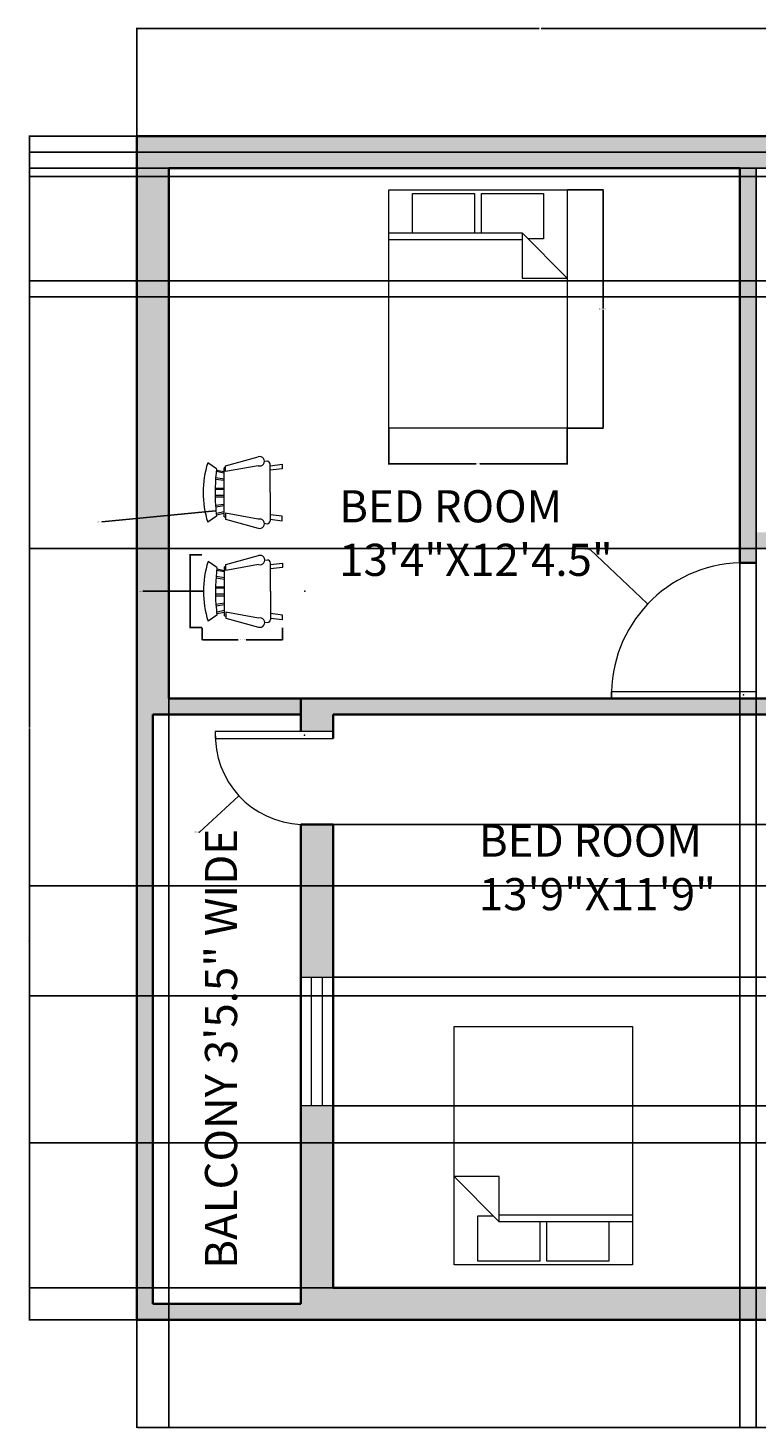
# Model space of a CAD drawing. Units: feet. Extents: x 1699 to 2359, y 1819 to 2211.
# Tile 1 of 4: x 1699 to 1903, y 1819 to 2211. Entities that reach past the tile are written whole.
import ezdxf

# ---------------------------------------------------------------- set-up
doc = ezdxf.new("R2010")
doc.units = ezdxf.units.FT
for name, color, linetype, lineweight in [('A-ANNO-DIMS', 2, 'Continuous', 18), ('A-AREA-IDEN', 7, 'Continuous', 18), ('A-DOOR', 4, 'Continuous', 18), ('A-FURN', 8, 'Continuous', 18), ('A-GLAZ', 3, 'Continuous', 18), ('A-WALL', 7, 'Continuous', 35), ('A-WALL-PATT', 1, 'Continuous', 13)]:
    doc.layers.add(name, color=color, linetype=linetype, lineweight=lineweight)
doc.styles.get("Standard").update_dxf_attribs({"font": 'arial.ttf'})
doc.dimstyles.get("Standard").update_dxf_attribs({"dimtxt": 0.18, "dimasz": 0.18, "dimexe": 0.18, "dimexo": 0.0625, "dimgap": 0.09, "dimtad": 0, "dimtih": 1, "dimtoh": 1, "dimdec": 4, "dimzin": 0, "dimdsep": 46, "dimtxsty": 'Standard', "dimcen": 0.09, "dimadec": 0, "dimazin": 0, "dimtfac": 1, "dimtdec": 4, "dimtofl": 0, "dimtmove": 0, "dimatfit": 3, "dimfxl": 1, "dimtolj": 1, "dimtzin": 0, "dimarcsym": 0})

# ---------------------------------------------------------------- blocks, each defined once
blk = doc.blocks.new('Bed - Queen')
for p, q in [((0, -80.00003), (0, 0)), ((0, 0), (59.99999, 0)), ((59.99999, 0), (59.99999, -80.00003)), ((7.99999, -1.2), (28.79998, -1.2)), ((7.99999, -14.4), (7.99999, -1.2)), ((28.79998, -1.2), (28.79998, -14.4)), ((31.19999, -1.2), (51.99999, -1.2)), ((31.19999, -14.4), (31.19999, -1.2)), ((51.99999, -1.2), (51.99999, -16.4)), ((0, -14.4), (44.8, -14.4)), ((44.8, -16.8), (0, -16.8)), ((59.99999, -29.6), (44.8, -14.4)), ((44.8, -14.4), (44.8, -29.6)), ((51.99999, -16.4), (46.79936, -16.4)), ((44.8, -29.6), (59.99999, -29.6)), ((59.99999, -80.00003), (0, -80.00003))]:
    blk.add_line(p, q)
blk = doc.blocks.new('Chair - Rocking')
for p, q in [((-8, -4.5), (-10, -1.5)), ((-7.5, -4.5), (-7, -7)), ((-6.5, -7), (-7.02225, -4.43)), ((-4.5, -7), (-4.96674, -4.19951)), ((-4, -7), (-4.40532, -4.16272)), ((-1.5, -4.05012), (-1.5, -7)), ((-1, -7), (-1, -4.05012)), ((1, -7), (1, -4.04655)), ((1.5, -4.05012), (1.5, -7)), ((4, -7), (4.40187, -4.18694)), ((4.5, -7), (4.96761, -4.19437)), ((6.5, -7), (7, -4.4057)), ((7.5, -4.5), (7, -7)), ((8, -4.5), (10, -1.5)), ((-9, -7.5), (-12, -18.49999)), ((-7, -7.5), (-9, -7.5)), ((-9, -18.49999), (-7, -7.5)), ((-8.23428, -6.99939), (-8.3093, -7.47958)), ((-8.23041, -7), (8.23915, -7)), ((7, -7.5), (9, -7.5)), ((9, -18.49999), (7, -7.5)), ((8.31071, -7.48854), (8.23449, -7.00073)), ((9, -7.5), (12, -18.49999)), ((-10.36644, -20.64523), (-10.5, -21.49999)), ((-9, -22.49999), (-9.5, -26.49999)), ((0, -22.49999), (-9.5, -22.49999)), ((-8, -26.49999), (-7.5, -22.49999)), ((0, -22.49999), (9.5, -22.49999)), ((8, -26.49999), (7.5, -22.49999)), ((9, -22.49999), (9.5, -26.49999)), ((10.5, -21.49999), (10.3575, -20.58798)), ((-9.5, -26.49999), (-8, -26.49999)), ((9.5, -26.49999), (8, -26.49999))]:
    blk.add_line(p, q)
for centre, radius, start, end in [((0, -34.08333), 34.08333, 72.93847, 107.0615), ((0, -68.25004), 64.25, 93.92211, 97.15267), ((0, -68.25004), 64.25, 82.84733, 93.92211), ((-10.5, -18.99999), 1.58114, 161.5651, 18.43495), ((10.5, -18.99999), 1.58114, 161.5651, 18.43495), ((-9.5, -21.49999), 1, 180, 270), ((9.5, -21.49999), 1, 270, 0)]:
    blk.add_arc(centre, radius, start, end)
blk = doc.blocks.new('DOOR-SWING-36')
for p, q in [((0.01, 0), (0.01, 2)), ((0.01, 2), (40.51, 2)), ((36.01, 0), (0.01, 0))]:
    blk.add_line(p, q)
blk.add_arc((37.01, 1), 37.01, 91.5482, 181.5482)
blk = doc.blocks.new('*D8')
at = {"layer": 'A-ANNO-DIMS', "color": 0, "lineweight": -2, "transparency": 16777216}
for p, q in [((1850.12, 2165.27), (1860.24, 2165.27)), ((1860.06, 2165.09), (1860.06, 2132.12)), ((1860.06, 2098.78), (1860.06, 2131.75)), ((1850.12, 2098.6), (1860.24, 2098.6))]:
    blk.add_line(p, q, dxfattribs=at)
at = {"layer": 'A-ANNO-DIMS', "color": 0, "transparency": 16777216}
for points in [[(1860.03, 2165.09), (1860.09, 2165.09), (1860.06, 2165.27)], [(1860.03, 2098.78), (1860.09, 2098.78), (1860.06, 2098.6)]]:
    blk.add_solid(points, dxfattribs=at)
at = {"layer": 'Defpoints', "color": 0, "transparency": 16777216}
for p in [(1850.06, 2165.27), (1860.06, 2165.27), (1850.06, 2098.6)]:
    blk.add_point(p, dxfattribs=at)
at = {"layer": 'A-ANNO-DIMS', "color": 0, "transparency": 16777216, "insert": (1860.06, 2131.93), "char_height": 0.18, "attachment_point": 5}
blk.add_mtext('\\A1;QUEEN BED 67 TYP.', dxfattribs=at)
blk = doc.blocks.new('*D9')
at = {"layer": 'A-ANNO-DIMS', "color": 0, "lineweight": -2, "transparency": 16777216}
for p, q in [((1800.06, 2098.54), (1800.06, 2088.42)), ((1850.06, 2098.54), (1850.06, 2088.42)), ((1800.24, 2088.6), (1824.53, 2088.6)), ((1849.88, 2088.6), (1825.59, 2088.6))]:
    blk.add_line(p, q, dxfattribs=at)
at = {"layer": 'A-ANNO-DIMS', "color": 0, "transparency": 16777216}
for points in [[(1800.24, 2088.63), (1800.24, 2088.57), (1800.06, 2088.6)], [(1849.88, 2088.63), (1849.88, 2088.57), (1850.06, 2088.6)]]:
    blk.add_solid(points, dxfattribs=at)
at = {"layer": 'Defpoints', "color": 0, "transparency": 16777216}
for p in [(1800.06, 2098.6), (1850.06, 2098.6), (1850.06, 2088.6)]:
    blk.add_point(p, dxfattribs=at)
at = {"layer": 'A-ANNO-DIMS', "color": 0, "transparency": 16777216, "insert": (1825.06, 2088.6), "char_height": 0.18, "attachment_point": 5}
blk.add_mtext('\\A1;50 TYP.', dxfattribs=at)
blk = doc.blocks.new('*D10')
at = {"layer": 'A-ANNO-DIMS', "color": 0, "lineweight": -2, "transparency": 16777216}
for p, q in [((1747.72, 2042.64), (1747.72, 2039.15)), ((1770.22, 2042.64), (1770.22, 2039.15)), ((1747.9, 2039.33), (1757.88, 2039.33)), ((1770.04, 2039.33), (1760.07, 2039.33))]:
    blk.add_line(p, q, dxfattribs=at)
at = {"layer": 'A-ANNO-DIMS', "color": 0, "transparency": 16777216}
for points in [[(1747.9, 2039.36), (1747.9, 2039.3), (1747.72, 2039.33)], [(1770.04, 2039.36), (1770.04, 2039.3), (1770.22, 2039.33)]]:
    blk.add_solid(points, dxfattribs=at)
at = {"layer": 'Defpoints', "color": 0, "transparency": 16777216}
for p in [(1747.72, 2042.7), (1770.22, 2042.7), (1747.72, 2039.33)]:
    blk.add_point(p, dxfattribs=at)
at = {"layer": 'A-ANNO-DIMS', "color": 0, "transparency": 16777216, "insert": (1758.97, 2039.33), "char_height": 0.18, "attachment_point": 5}
blk.add_mtext('\\A1;ROCKER 22 TYP.', dxfattribs=at)
blk = doc.blocks.new('*D11')
at = {"layer": 'A-ANNO-DIMS', "color": 0, "lineweight": -2, "transparency": 16777216}
for p, q in [((1747.66, 2063.06), (1744.17, 2063.06)), ((1744.35, 2062.88), (1744.35, 2053.06)), ((1744.35, 2042.88), (1744.35, 2052.7)), ((1747.66, 2042.7), (1744.17, 2042.7))]:
    blk.add_line(p, q, dxfattribs=at)
at = {"layer": 'A-ANNO-DIMS', "color": 0, "transparency": 16777216}
for points in [[(1744.32, 2062.88), (1744.38, 2062.88), (1744.35, 2063.06)], [(1744.32, 2042.88), (1744.38, 2042.88), (1744.35, 2042.7)]]:
    blk.add_solid(points, dxfattribs=at)
at = {"layer": 'Defpoints', "color": 0, "transparency": 16777216}
for p in [(1744.35, 2063.06), (1747.72, 2063.06), (1747.72, 2042.7)]:
    blk.add_point(p, dxfattribs=at)
at = {"layer": 'A-ANNO-DIMS', "color": 0, "transparency": 16777216, "insert": (1744.35, 2052.88), "char_height": 0.18, "attachment_point": 5}
blk.add_mtext('\\A1;20 TYP.', dxfattribs=at)
blk = doc.blocks.new('*D25')
at = {"layer": 'A-ANNO-DIMS', "color": 0, "lineweight": -2, "transparency": 16777216}
for p, q in [((1729.43, 2180.29), (1729.43, 1818.57)), ((1738.43, 2171.29), (1738.43, 1818.57)), ((1729.61, 1818.75), (1733.78, 1818.75)), ((1738.25, 1818.75), (1734.08, 1818.75))]:
    blk.add_line(p, q, dxfattribs=at)
at = {"layer": 'A-ANNO-DIMS', "color": 0, "transparency": 16777216}
for points in [[(1729.61, 1818.78), (1729.61, 1818.72), (1729.43, 1818.75)], [(1738.25, 1818.78), (1738.25, 1818.72), (1738.43, 1818.75)]]:
    blk.add_solid(points, dxfattribs=at)
at = {"layer": 'Defpoints', "color": 0, "transparency": 16777216}
for p in [(1729.43, 2180.35), (1738.43, 2171.35), (1729.43, 1818.75)]:
    blk.add_point(p, dxfattribs=at)
at = {"layer": 'A-ANNO-DIMS', "color": 0, "transparency": 16777216, "insert": (1733.93, 1818.75), "char_height": 0.18, "attachment_point": 5}
blk.add_mtext('\\A1;9', dxfattribs=at)
blk = doc.blocks.new('*D27')
at = {"layer": 'A-ANNO-DIMS', "color": 0, "lineweight": -2, "transparency": 16777216}
for p, q in [((2114.36, 2175.85), (1699.15, 2175.85)), ((1699.33, 2175.67), (1699.33, 2158.03)), ((1699.33, 2140.03), (1699.33, 2157.67)), ((2114.36, 2139.85), (1699.15, 2139.85))]:
    blk.add_line(p, q, dxfattribs=at)
at = {"layer": 'A-ANNO-DIMS', "color": 0, "transparency": 16777216}
for points in [[(1699.3, 2175.67), (1699.36, 2175.67), (1699.33, 2175.85)], [(1699.3, 2140.03), (1699.36, 2140.03), (1699.33, 2139.85)]]:
    blk.add_solid(points, dxfattribs=at)
at = {"layer": 'Defpoints', "color": 0, "transparency": 16777216}
for p in [(2114.43, 2175.85), (1699.33, 2139.85), (2114.43, 2139.85)]:
    blk.add_point(p, dxfattribs=at)
at = {"layer": 'A-ANNO-DIMS', "color": 0, "transparency": 16777216, "insert": (1699.33, 2157.85), "char_height": 0.18, "attachment_point": 5}
blk.add_mtext('\\A1;36', dxfattribs=at)
blk = doc.blocks.new('*D38')
at = {"layer": 'A-ANNO-DIMS', "color": 0, "lineweight": -2, "transparency": 16777216}
for p, q in [((1784.49, 1944.78), (2359.21, 1944.78)), ((2359.03, 1944.6), (2359.03, 1926.96)), ((2359.03, 1908.96), (2359.03, 1926.6)), ((1784.49, 1908.78), (2359.21, 1908.78))]:
    blk.add_line(p, q, dxfattribs=at)
at = {"layer": 'A-ANNO-DIMS', "color": 0, "transparency": 16777216}
for points in [[(2359, 1944.6), (2359.06, 1944.6), (2359.03, 1944.78)], [(2359, 1908.96), (2359.06, 1908.96), (2359.03, 1908.78)]]:
    blk.add_solid(points, dxfattribs=at)
at = {"layer": 'Defpoints', "color": 0, "transparency": 16777216}
for p in [(1784.43, 1944.78), (2359.03, 1944.78), (1784.43, 1908.78)]:
    blk.add_point(p, dxfattribs=at)
at = {"layer": 'A-ANNO-DIMS', "color": 0, "transparency": 16777216, "insert": (2359.03, 1926.78), "char_height": 0.18, "attachment_point": 5}
blk.add_mtext('\\A1;36', dxfattribs=at)
blk = doc.blocks.new('*D39')
at = {"layer": 'A-ANNO-DIMS', "color": 0, "lineweight": -2, "transparency": 16777216}
for p, q in [((1784.49, 1987.61), (2359.21, 1987.61)), ((2359.03, 1987.43), (2359.03, 1966.38)), ((2359.03, 1944.96), (2359.03, 1966.02)), ((1784.49, 1944.78), (2359.21, 1944.78))]:
    blk.add_line(p, q, dxfattribs=at)
at = {"layer": 'A-ANNO-DIMS', "color": 0, "transparency": 16777216}
for points in [[(2359, 1987.43), (2359.06, 1987.43), (2359.03, 1987.61)], [(2359, 1944.96), (2359.06, 1944.96), (2359.03, 1944.78)]]:
    blk.add_solid(points, dxfattribs=at)
at = {"layer": 'Defpoints', "color": 0, "transparency": 16777216}
for p in [(1784.43, 1987.61), (2359.03, 1987.61), (1784.43, 1944.78)]:
    blk.add_point(p, dxfattribs=at)
at = {"layer": 'A-ANNO-DIMS', "color": 0, "transparency": 16777216, "insert": (2359.03, 1966.2), "char_height": 0.18, "attachment_point": 5}
blk.add_mtext('\\A1;42.83', dxfattribs=at)
blk = doc.blocks.new('*D40')
at = {"layer": 'A-ANNO-DIMS', "color": 0, "lineweight": -2, "transparency": 16777216}
for p, q in [((1729.43, 1848.79), (1729.43, 1818.57)), ((2328.93, 1848.79), (2328.93, 1818.57)), ((1729.61, 1818.75), (2028.78, 1818.75)), ((2328.75, 1818.75), (2029.57, 1818.75))]:
    blk.add_line(p, q, dxfattribs=at)
at = {"layer": 'A-ANNO-DIMS', "color": 0, "transparency": 16777216}
for points in [[(1729.61, 1818.78), (1729.61, 1818.72), (1729.43, 1818.75)], [(2328.75, 1818.78), (2328.75, 1818.72), (2328.93, 1818.75)]]:
    blk.add_solid(points, dxfattribs=at)
at = {"layer": 'Defpoints', "color": 0, "transparency": 16777216}
for p in [(1729.43, 1848.85), (2328.93, 1848.85), (2328.93, 1818.75)]:
    blk.add_point(p, dxfattribs=at)
at = {"layer": 'A-ANNO-DIMS', "color": 0, "transparency": 16777216, "insert": (2029.18, 1818.75), "char_height": 0.18, "attachment_point": 5}
blk.add_mtext('\\A1;599.5', dxfattribs=at)
blk = doc.blocks.new('*D41')
at = {"layer": 'A-ANNO-DIMS', "color": 0, "lineweight": -2, "transparency": 16777216}
for p, q in [((1729.36, 2180.35), (1699.15, 2180.35)), ((1699.33, 2180.17), (1699.33, 2014.78)), ((1699.33, 1849.03), (1699.33, 2014.42)), ((1729.36, 1848.85), (1699.15, 1848.85))]:
    blk.add_line(p, q, dxfattribs=at)
at = {"layer": 'A-ANNO-DIMS', "color": 0, "transparency": 16777216}
for points in [[(1699.3, 2180.17), (1699.36, 2180.17), (1699.33, 2180.35)], [(1699.3, 1849.03), (1699.36, 1849.03), (1699.33, 1848.85)]]:
    blk.add_solid(points, dxfattribs=at)
at = {"layer": 'Defpoints', "color": 0, "transparency": 16777216}
for p in [(1699.33, 2180.35), (1729.43, 2180.35), (1729.43, 1848.85)]:
    blk.add_point(p, dxfattribs=at)
at = {"layer": 'A-ANNO-DIMS', "color": 0, "transparency": 16777216, "insert": (1699.33, 2014.6), "char_height": 0.18, "attachment_point": 5}
blk.add_mtext('\\A1;331.5', dxfattribs=at)
blk = doc.blocks.new('*D43')
at = {"layer": 'A-ANNO-DIMS', "color": 0, "lineweight": -2, "transparency": 16777216}
for p, q in [((1991.36, 1898.47), (1699.15, 1898.47)), ((1699.33, 1898.29), (1699.33, 1878.34)), ((1699.33, 1858.03), (1699.33, 1877.98)), ((1991.36, 1857.85), (1699.15, 1857.85))]:
    blk.add_line(p, q, dxfattribs=at)
at = {"layer": 'A-ANNO-DIMS', "color": 0, "transparency": 16777216}
for points in [[(1699.3, 1898.29), (1699.36, 1898.29), (1699.33, 1898.47)], [(1699.3, 1858.03), (1699.36, 1858.03), (1699.33, 1857.85)]]:
    blk.add_solid(points, dxfattribs=at)
at = {"layer": 'Defpoints', "color": 0, "transparency": 16777216}
for p in [(1991.43, 1898.47), (1699.33, 1857.85), (1991.43, 1857.85)]:
    blk.add_point(p, dxfattribs=at)
at = {"layer": 'A-ANNO-DIMS', "color": 0, "transparency": 16777216, "insert": (1699.33, 1878.16), "char_height": 0.18, "attachment_point": 5}
blk.add_mtext('\\A1;40.62', dxfattribs=at)
blk = doc.blocks.new('*D46')
at = {"layer": 'A-ANNO-DIMS', "color": 0, "lineweight": -2, "transparency": 16777216}
for p, q in [((2013.86, 2135.35), (1699.15, 2135.35)), ((1699.33, 2135.17), (1699.33, 2100.28)), ((1699.33, 2065.03), (1699.33, 2099.92)), ((2013.86, 2064.85), (1699.15, 2064.85))]:
    blk.add_line(p, q, dxfattribs=at)
at = {"layer": 'A-ANNO-DIMS', "color": 0, "transparency": 16777216}
for points in [[(1699.3, 2135.17), (1699.36, 2135.17), (1699.33, 2135.35)], [(1699.3, 2065.03), (1699.36, 2065.03), (1699.33, 2064.85)]]:
    blk.add_solid(points, dxfattribs=at)
at = {"layer": 'Defpoints', "color": 0, "transparency": 16777216}
for p in [(1699.33, 2135.35), (2013.93, 2135.35), (2013.93, 2064.85)]:
    blk.add_point(p, dxfattribs=at)
at = {"layer": 'A-ANNO-DIMS', "color": 0, "transparency": 16777216, "insert": (1699.33, 2100.1), "char_height": 0.18, "attachment_point": 5}
blk.add_mtext('\\A1;70.5', dxfattribs=at)
blk = doc.blocks.new('*D47')
at = {"layer": 'A-ANNO-DIMS', "color": 0, "lineweight": -2, "transparency": 16777216}
for p, q in [((1898.43, 2171.29), (1898.43, 1818.57)), ((1902.93, 2171.29), (1902.93, 1818.57)), ((1898.61, 1818.75), (1900.42, 1818.75)), ((1902.75, 1818.75), (1900.93, 1818.75))]:
    blk.add_line(p, q, dxfattribs=at)
at = {"layer": 'A-ANNO-DIMS', "color": 0, "transparency": 16777216}
for points in [[(1898.61, 1818.78), (1898.61, 1818.72), (1898.43, 1818.75)], [(1902.75, 1818.78), (1902.75, 1818.72), (1902.93, 1818.75)]]:
    blk.add_solid(points, dxfattribs=at)
at = {"layer": 'Defpoints', "color": 0, "transparency": 16777216}
for p in [(1898.43, 2171.35), (1902.93, 2171.35), (1902.93, 1818.75)]:
    blk.add_point(p, dxfattribs=at)
at = {"layer": 'A-ANNO-DIMS', "color": 0, "transparency": 16777216, "insert": (1900.68, 1818.75), "char_height": 0.18, "attachment_point": 5}
blk.add_mtext('\\A1;4.5', dxfattribs=at)
blk = doc.blocks.new('*D48')
at = {"layer": 'A-ANNO-DIMS', "color": 0, "lineweight": -2, "transparency": 16777216}
for p, q in [((2180.36, 1970.41), (1699.15, 1970.41)), ((1699.33, 1970.23), (1699.33, 1955.18)), ((1699.33, 1939.76), (1699.33, 1954.81)), ((2180.36, 1939.58), (1699.15, 1939.58))]:
    blk.add_line(p, q, dxfattribs=at)
at = {"layer": 'A-ANNO-DIMS', "color": 0, "transparency": 16777216}
for points in [[(1699.3, 1970.23), (1699.36, 1970.23), (1699.33, 1970.41)], [(1699.3, 1939.76), (1699.36, 1939.76), (1699.33, 1939.58)]]:
    blk.add_solid(points, dxfattribs=at)
at = {"layer": 'Defpoints', "color": 0, "transparency": 16777216}
for p in [(1699.33, 1970.41), (2180.43, 1970.41), (2180.43, 1939.58)]:
    blk.add_point(p, dxfattribs=at)
at = {"layer": 'A-ANNO-DIMS', "color": 0, "transparency": 16777216, "insert": (1699.33, 1954.99), "char_height": 0.18, "attachment_point": 5}
blk.add_mtext('\\A1;30.833', dxfattribs=at)
blk = doc.blocks.new('*D50')
at = {"layer": 'A-ANNO-DIMS', "color": 0, "lineweight": -2, "transparency": 16777216}
for p, q in [((1950.86, 2171.35), (1699.15, 2171.35)), ((1950.86, 2169.04), (1699.15, 2169.04)), ((1699.33, 2171.17), (1699.33, 2170.38)), ((1699.33, 2169.22), (1699.33, 2170.01))]:
    blk.add_line(p, q, dxfattribs=at)
at = {"layer": 'A-ANNO-DIMS', "color": 0, "transparency": 16777216}
for points in [[(1699.3, 2171.17), (1699.36, 2171.17), (1699.33, 2171.35)], [(1699.3, 2169.22), (1699.36, 2169.22), (1699.33, 2169.04)]]:
    blk.add_solid(points, dxfattribs=at)
at = {"layer": 'Defpoints', "color": 0, "transparency": 16777216}
for p in [(1699.33, 2169.04), (1950.93, 2171.35), (1950.93, 2169.04)]:
    blk.add_point(p, dxfattribs=at)
at = {"layer": 'A-ANNO-DIMS', "color": 0, "transparency": 16777216, "insert": (1699.33, 2170.19), "char_height": 0.18, "attachment_point": 5}
blk.add_mtext('\\A1;2.312', dxfattribs=at)
blk = doc.blocks.new('*D52')
at = {"layer": 'A-ANNO-DIMS', "color": 0, "lineweight": -2, "transparency": 16777216}
for p, q in [((1729.43, 2180.41), (1729.43, 2210.63)), ((1729.61, 2210.45), (1842.14, 2210.45)), ((1955.25, 2210.45), (1842.72, 2210.45)), ((1955.43, 2175.91), (1955.43, 2210.63))]:
    blk.add_line(p, q, dxfattribs=at)
at = {"layer": 'A-ANNO-DIMS', "color": 0, "transparency": 16777216}
for points in [[(1729.61, 2210.48), (1729.61, 2210.42), (1729.43, 2210.45)], [(1955.25, 2210.48), (1955.25, 2210.42), (1955.43, 2210.45)]]:
    blk.add_solid(points, dxfattribs=at)
at = {"layer": 'Defpoints', "color": 0, "transparency": 16777216}
for p in [(1955.43, 2210.45), (1729.43, 2180.35), (1955.43, 2175.85)]:
    blk.add_point(p, dxfattribs=at)
at = {"layer": 'A-ANNO-DIMS', "color": 0, "transparency": 16777216, "insert": (1842.43, 2210.45), "char_height": 0.18, "attachment_point": 5}
blk.add_mtext('\\A1;226', dxfattribs=at)
blk = doc.blocks.new('*D53')
at = {"layer": 'A-ANNO-DIMS', "color": 0, "lineweight": -2, "transparency": 16777216}
for p, q in [((1856.25, 2064.58), (1856.43, 2064.58)), ((1856.43, 2064.58), (1872.43, 2049.43)), ((1899.34, 2023.85), (1899.52, 2023.85)), ((1899.43, 2023.76), (1899.43, 2023.94))]:
    blk.add_line(p, q, dxfattribs=at)
at = {"layer": 'A-ANNO-DIMS', "color": 0, "transparency": 16777216}
blk.add_solid([(1872.45, 2049.45), (1872.41, 2049.41), (1872.56, 2049.31)], dxfattribs=at)
at = {"layer": 'Defpoints', "color": 0, "transparency": 16777216}
for p in [(1872.56, 2049.31), (1899.43, 2023.85)]:
    blk.add_point(p, dxfattribs=at)
at = {"layer": 'A-ANNO-DIMS', "color": 0, "transparency": 16777216, "insert": (1855.6, 2064.58), "char_height": 0.18, "attachment_point": 5}
blk.add_mtext('\\A1;2X R37.01', dxfattribs=at)
blk = doc.blocks.new('*D54')
at = {"layer": 'A-ANNO-DIMS', "color": 0, "lineweight": -2, "transparency": 16777216}
for p, q in [((1776.34, 2012.61), (1776.52, 2012.61)), ((1776.43, 2012.52), (1776.43, 2012.7)), ((1747.01, 1985.46), (1757.91, 1995.52)), ((1746.83, 1985.46), (1747.01, 1985.46))]:
    blk.add_line(p, q, dxfattribs=at)
at = {"layer": 'A-ANNO-DIMS', "color": 0, "transparency": 16777216}
blk.add_solid([(1757.89, 1995.54), (1757.93, 1995.5), (1758.04, 1995.64)], dxfattribs=at)
at = {"layer": 'Defpoints', "color": 0, "transparency": 16777216}
for p in [(1776.43, 2012.61), (1758.04, 1995.64)]:
    blk.add_point(p, dxfattribs=at)
at = {"layer": 'A-ANNO-DIMS', "color": 0, "transparency": 16777216, "insert": (1746.16, 1985.46), "char_height": 0.18, "attachment_point": 5}
blk.add_mtext('\\A1;4X R25.02', dxfattribs=at)
blk = doc.blocks.new('*D61')
at = {"layer": 'A-ANNO-DIMS', "color": 0, "lineweight": -2, "transparency": 16777216}
for p, q in [((1804.83, 2080.56), (1805.01, 2080.56)), ((1804.92, 2080.47), (1804.92, 2080.65)), ((1719.65, 2072.29), (1751.45, 2075.37))]:
    blk.add_line(p, q, dxfattribs=at)
at = {"layer": 'A-ANNO-DIMS', "color": 0, "transparency": 16777216}
blk.add_solid([(1751.45, 2075.4), (1751.45, 2075.34), (1751.63, 2075.39)], dxfattribs=at)
at = {"layer": 'Defpoints', "color": 0, "transparency": 16777216}
for p in [(1804.92, 2080.56), (1751.63, 2075.39)]:
    blk.add_point(p, dxfattribs=at)
at = {"layer": 'A-ANNO-DIMS', "color": 0, "transparency": 16777216, "insert": (1718.98, 2072.29), "char_height": 0.18, "attachment_point": 5}
blk.add_mtext('\\A1;4X R53.54', dxfattribs=at)
blk = doc.blocks.new('*D62')
at = {"layer": 'A-ANNO-DIMS', "color": 0, "lineweight": -2, "transparency": 16777216}
for p, q in [((1731.1, 2052.88), (1747.96, 2052.88)), ((1776.45, 2052.88), (1776.63, 2052.88)), ((1776.54, 2052.79), (1776.54, 2052.97))]:
    blk.add_line(p, q, dxfattribs=at)
at = {"layer": 'A-ANNO-DIMS', "color": 0, "transparency": 16777216}
blk.add_solid([(1747.96, 2052.91), (1747.96, 2052.85), (1748.14, 2052.88)], dxfattribs=at)
at = {"layer": 'Defpoints', "color": 0, "transparency": 16777216}
for p in [(1748.14, 2052.88), (1776.54, 2052.88)]:
    blk.add_point(p, dxfattribs=at)
at = {"layer": 'A-ANNO-DIMS', "color": 0, "transparency": 16777216, "insert": (1730.49, 2052.88), "char_height": 0.18, "attachment_point": 5}
blk.add_mtext('\\A1;2X R28.4', dxfattribs=at)

msp = doc.modelspace()

# ---------------------------------------------------------------- hatches: boundary and pattern name
at = {"layer": 'A-WALL-PATT'}
h = msp.add_hatch(color=256, dxfattribs=at)
h.dxf.hatch_style = 1
h.paths.add_polyline_path([(2180.4267, 1853.3494), (2180.4267, 1857.8494), (1955.4267, 1857.8494), (1955.4267, 1935.0782), (1991.4267, 1935.0782), (1991.4267, 1939.5782), (1955.4267, 1939.5782), (1955.4267, 2022.8494), (1950.9267, 2022.8494), (1950.9267, 1857.8494), (1784.4267, 1857.8494), (1784.4267, 1908.7829), (1775.4267, 1908.7829), (1775.4267, 1853.3494), (1733.9267, 1853.3494), (1733.9267, 2018.3494), (1775.4267, 2018.3494), (1775.4267, 2022.8494), (1738.4267, 2022.8494), (1738.4267, 2171.3494), (1898.4267, 2171.3494), (1898.4267, 2060.8494), (1902.9267, 2060.8494), (1902.9267, 2064.8494), (1955.4267, 2064.8494), (1955.4267, 2069.3494), (1902.9267, 2069.3494), (1902.9267, 2171.3494), (1950.9267, 2171.3494), (1950.9267, 2169.0373), (1955.4267, 2169.0373), (1955.4267, 2175.8494), (2114.4267, 2175.8494), (2114.4267, 2167.1408), (2118.9267, 2167.1408), (2118.9267, 2171.3494), (2166.9267, 2171.3494), (2166.9267, 2113.3494), (2171.4267, 2113.3494), (2171.4267, 2171.3494), (2319.9267, 2171.3494), (2319.9267, 2132.5785), (2328.9267, 2132.5785), (2328.9267, 2180.3494), (2309.4267, 2180.3494), (1729.4267, 2180.3494), (1729.4267, 1848.8494), (2180.4267, 1848.8494)])
h.paths.add_polyline_path([(1784.4267, 1987.6139), (1775.4267, 1987.6139), (1775.4267, 1944.7829), (1784.4267, 1944.7829)], flags=17)
h.paths.add_polyline_path([(1912.9267, 2022.8494), (1775.4267, 2022.8494), (1775.4267, 2013.6139), (1784.4267, 2013.6139), (1784.4267, 2018.3494), (1912.9267, 2018.3494)], flags=17)
h.paths.add_polyline_path([(2018.4267, 2135.3494), (2047.4307, 2135.3494), (2047.4307, 2139.8494), (1981.4267, 2139.8494), (1981.4267, 2135.3494), (2013.9267, 2135.3494), (2013.9267, 2059.8494), (2018.4267, 2059.8494)], flags=17)
h.paths.add_polyline_path([(2114.4267, 2139.8494), (2071.4307, 2139.8494), (2071.4307, 2135.3494), (2114.4267, 2135.3494)], flags=17)
h.paths.add_polyline_path([(2118.9267, 2143.1408), (2114.4267, 2143.1408), (2114.4267, 2059.8494), (2118.9267, 2059.8494), (2118.9267, 2082.8494), (2184.631, 2082.8494), (2184.631, 2087.3494), (2118.9267, 2087.3494)], flags=17)
h.paths.add_polyline_path([(2328.9267, 2084.5785), (2319.9267, 2084.5785), (2319.9267, 2022.8494), (2232.7955, 2022.8494), (2232.7955, 2013.3494), (2319.9267, 2013.3494), (2319.9267, 1998.3723), (2328.9267, 1998.3723)], flags=17)
h.paths.add_polyline_path([(2180.4267, 2043.5261), (2171.4267, 2043.5261), (2171.4267, 2006.4114), (2180.4267, 2006.4114)], flags=17)
h.paths.add_polyline_path([(2015.0526, 1939.5782), (1991.4267, 1939.5782), (1991.4267, 1935.0782), (2015.0526, 1935.0782)], flags=17)
h.paths.add_polyline_path([(2180.4267, 1939.5782), (2087.0526, 1939.5782), (2087.0526, 1935.0782), (2180.4267, 1935.0782)], flags=17)
h.paths.add_polyline_path([(2328.9267, 1868.1839), (2319.9267, 1868.1839), (2319.9267, 1853.3494), (2180.4267, 1853.3494), (2180.4267, 1848.8494), (2328.9267, 1848.8494)], flags=17)

# ---------------------------------------------------------------- linework, layer by layer
at = {"layer": 'A-DOOR'}
for p, q in [((1784.4267, 2013.6139), (1751.4267, 2013.6139)), ((1775.4267, 2013.6139), (1751.4267, 2013.6139)), ((1751.4267, 2013.6139), (1751.4267, 2011.6139)), ((1751.4267, 2011.6139), (1784.4267, 2011.6139))]:
    msp.add_line(p, q, dxfattribs=at)
msp.add_arc((1776.4267, 2012.6139), 25.02, 177.70939, 267.70939, dxfattribs=at)
at = {"layer": 'A-GLAZ'}
for p, q in [((1775.4267, 1944.7829), (1784.4267, 1944.7829)), ((1775.4267, 1908.7829), (1775.4267, 1944.7829)), ((1778.4267, 1908.7829), (1778.4267, 1944.7829)), ((1781.4267, 1908.7829), (1781.4267, 1944.7829)), ((1784.4267, 1944.7829), (1784.4267, 1908.7829)), ((1784.4267, 1908.7829), (1775.4267, 1908.7829))]:
    msp.add_line(p, q, dxfattribs=at)
at = {"layer": 'A-WALL'}
for p, q in [((1729.4267, 2180.3494), (2309.4267, 2180.3494)), ((1729.4267, 2180.3494), (1729.4267, 1848.8494)), ((1738.4267, 2171.3494), (1898.4267, 2171.3494)), ((1738.4267, 2171.3494), (1738.4267, 2022.8494)), ((1898.4267, 2171.3494), (1898.4267, 2060.8494)), ((1902.9267, 2060.8494), (1898.4267, 2060.8494)), ((1738.4267, 2022.8494), (1912.9267, 2022.8494)), ((1775.4267, 2022.8494), (1775.4267, 2013.6139)), ((1733.9267, 2018.3494), (1775.4267, 2018.3494)), ((1733.9267, 2018.3494), (1733.9267, 1853.3494)), ((1784.4267, 2018.3494), (1784.4267, 2011.6139)), ((1784.4267, 2018.3494), (1912.9267, 2018.3494)), ((1784.4267, 1987.6139), (1775.4267, 1987.6139)), ((1775.4267, 1987.6139), (1775.4267, 1853.3494)), ((1784.4267, 1987.6139), (1784.4267, 1857.8494)), ((1784.4267, 1857.8494), (1950.9267, 1857.8494)), ((1733.9267, 1853.3494), (1775.4267, 1853.3494)), ((1729.4267, 1848.8494), (2328.9267, 1848.8494))]:
    msp.add_line(p, q, dxfattribs=at)

# ---------------------------------------------------------------- block references
at = {"layer": 'A-DOOR'}
msp.add_blockref('DOOR-SWING-36', (1862.413, 2022.849), dxfattribs=at)
at = {"layer": 'A-FURN', "xscale": 0.8333333333333331, "yscale": 0.8333333333333331, "zscale": 0.8333333333333331}
msp.add_blockref('Bed - Queen', (1800.0612, 2165.2673), dxfattribs=at)
for name, p, rotation in [('Chair - Rocking', (1748.0445, 2080.5558), 90), ('Chair - Rocking', (1748.1387, 2052.8827), 90), ('Bed - Queen', (1868.3233, 1864.3022), 180)]:
    msp.add_blockref(name, p, dxfattribs=dict(at, rotation=rotation))

# ---------------------------------------------------------------- texts
at = {"layer": 'A-AREA-IDEN', "char_height": 9, "attachment_point": 1}
for s, width, insert in [('{\\fCambria|b0|i0|c0|p18;BED ROOM\\P13\'4"X12\'4.5"}', 113.284378, (1786.1423, 2081.1955)), ('{\\fCambria|b0|i0|c0|p18;BED ROOM\\P13\'9"X11\'9"}', 73.785518, (1825.2944, 1987.5686))]:
    msp.add_mtext_dynamic_manual_height_columns(s, width=width, gutter_width=12.5, heights=[0], dxfattribs=dict(at, insert=insert))
at = {"layer": 'A-AREA-IDEN', "insert": (1748.5398, 1863.17), "char_height": 9, "attachment_point": 1, "rotation": 90}
msp.add_mtext_dynamic_manual_height_columns('{\\fCambria|b0|i0|c0|p18;BALCONY 3\'5.5" WIDE}', width=131.719476, gutter_width=12.5, heights=[0], dxfattribs=at)

# ---------------------------------------------------------------- dimensions: what is measured, and where the dimension line sits
at = {"layer": 'A-ANNO-DIMS'}
for base, p1, p2, override, picture, middle in [((1955.4267, 2210.4494), (1729.4267, 2180.3494), (1955.4267, 2175.8494), {"dimdec": 0, "dimlfac": 1, "dimrnd": 0, "dimzin": 0, "dimdsep": 46, "dimlunit": 2}, '*D52', (1842.4267, 2210.4494)), ((1729.4267, 1818.7494), (1738.4267, 2171.3494), (1729.4267, 2180.3494), {"dimdec": 0, "dimlfac": 1, "dimrnd": 0, "dimzin": 0, "dimdsep": 46, "dimlunit": 2}, '*D25', (1733.9267, 1818.7494)), ((1902.9267, 1818.7494), (1898.4267, 2171.3494), (1902.9267, 2171.3494), {"dimdec": 1, "dimlfac": 1, "dimrnd": 0, "dimzin": 0, "dimdsep": 46, "dimlunit": 2}, '*D47', (1900.6767, 1818.7494)), ((2328.9267, 1818.7494), (1729.4267, 1848.8494), (2328.9267, 1848.8494), {"dimdec": 1, "dimlfac": 1, "dimrnd": 0, "dimzin": 0, "dimdsep": 46, "dimlunit": 2}, '*D40', (2029.1767, 1818.7494))]:
    dim = msp.add_linear_dim(base=base, p1=p1, p2=p2, dimstyle='Standard', override=override, dxfattribs=at)
    dim.commit()
    dim.dimension.update_dxf_attribs({"geometry": picture, "text_midpoint": middle})
for base, p1, p2, override, picture, middle in [((1699.3267, 2180.3494), (1729.4267, 1848.8494), (1729.4267, 2180.3494), {"dimdec": 1, "dimlfac": 1, "dimrnd": 0, "dimzin": 0, "dimdsep": 46, "dimlunit": 2}, '*D41', (1699.3267, 2014.5994)), ((1699.3267, 2139.8494), (2114.4267, 2175.8494), (2114.4267, 2139.8494), {"dimdec": 0, "dimlfac": 1, "dimrnd": 0, "dimzin": 0, "dimdsep": 46, "dimlunit": 2}, '*D27', (1699.3267, 2157.8494)), ((1699.3267, 2169.0373), (1950.9267, 2171.3494), (1950.9267, 2169.0373), {"dimdec": 3, "dimlfac": 1, "dimrnd": 0, "dimzin": 0, "dimdsep": 46, "dimlunit": 2}, '*D50', (1699.3267, 2170.1933)), ((1699.3267, 2135.3494), (2013.9267, 2064.8494), (2013.9267, 2135.3494), {"dimdec": 1, "dimlfac": 1, "dimrnd": 0, "dimzin": 0, "dimdsep": 46, "dimlunit": 2}, '*D46', (1699.3267, 2100.0994)), ((2359.0267, 1987.6139), (1784.4267, 1944.7829), (1784.4267, 1987.6139), {"dimdec": 2, "dimlfac": 1, "dimrnd": 0, "dimzin": 0, "dimdsep": 46, "dimlunit": 2}, '*D39', (2359.0267, 1966.1984)), ((1699.3267, 1970.4114), (2180.4267, 1939.5782), (2180.4267, 1970.4114), {"dimdec": 3, "dimlfac": 1, "dimrnd": 0, "dimzin": 0, "dimdsep": 46, "dimlunit": 2}, '*D48', (1699.3267, 1954.9948)), ((2359.0267, 1944.7829), (1784.4267, 1908.7829), (1784.4267, 1944.7829), {"dimdec": 0, "dimlfac": 1, "dimrnd": 0, "dimzin": 0, "dimdsep": 46, "dimlunit": 2}, '*D38', (2359.0267, 1926.7829)), ((1699.3267, 1857.8494), (1991.4267, 1898.4702), (1991.4267, 1857.8494), {"dimdec": 2, "dimlfac": 1, "dimrnd": 0, "dimzin": 0, "dimdsep": 46, "dimlunit": 2}, '*D43', (1699.3267, 1878.1598))]:
    dim = msp.add_linear_dim(base=base, p1=p1, p2=p2, angle=90, dimstyle='Standard', override=override, dxfattribs=at)
    dim.commit()
    dim.dimension.update_dxf_attribs({"geometry": picture, "text_midpoint": middle})
for base, p1, p2, angle, text, picture, middle in [((1860.0612, 2165.2673), (1850.0612, 2098.6006), (1850.0612, 2165.2673), 90, 'QUEEN BED <> TYP.', '*D8', (1860.0612, 2131.9339)), ((1744.347, 2063.064), (1747.722, 2042.7014), (1747.722, 2063.064), 90, '<> TYP.', '*D11', (1744.347, 2052.8827)), ((1747.72202, 2039.32643), (1770.22201, 2042.70143), (1747.72202, 2042.70143), 180, 'ROCKER <> TYP.', '*D10', (1758.97201, 2039.32643))]:
    dim = msp.add_linear_dim(base=base, p1=p1, p2=p2, angle=angle, text=text, dimstyle='Standard', override={"dimdec": 0, "dimlfac": 1, "dimrnd": 0, "dimzin": 0, "dimdsep": 46, "dimlunit": 2}, dxfattribs=at)
    dim.commit()
    dim.dimension.update_dxf_attribs({"geometry": picture, "text_midpoint": middle})
dim = msp.add_linear_dim(base=(1850.0612, 2088.6006), p1=(1800.0612, 2098.6006), p2=(1850.0612, 2098.6006), text='<> TYP.', dimstyle='Standard', override={"dimdec": 0, "dimlfac": 1, "dimrnd": 0, "dimzin": 0, "dimdsep": 46, "dimlunit": 2}, dxfattribs=at)
dim.commit()
dim.dimension.update_dxf_attribs({"geometry": '*D9', "text_midpoint": (1825.0612, 2088.6006)})
for center, mpoint, text, override, picture, middle in [((1804.9195, 2080.5558), (1751.6277, 2075.389), '4X <>', {"dimdec": 2, "dimlfac": 1, "dimrnd": 0, "dimzin": 0, "dimdsep": 46, "dimlunit": 2}, '*D61', (1719.6526, 2072.2889)), ((1899.4267, 2023.8494), (1872.5567, 2049.3053), '2X <>', {"dimdec": 2, "dimlfac": 1, "dimrnd": 0, "dimzin": 0, "dimdsep": 46, "dimlunit": 2}, '*D53', (1855.5973, 2064.5789)), ((1776.5415, 2052.8827), (1748.1387, 2052.883), '2X <>', {"dimdec": 1, "dimlfac": 1, "dimrnd": 0, "dimzin": 0, "dimdsep": 46, "dimlunit": 2}, '*D62', (1731.097, 2052.8832)), ((1776.4267, 2012.6139), (1758.0421, 1995.6431), '4X <>', {"dimdec": 2, "dimlfac": 1, "dimrnd": 0, "dimzin": 0, "dimdsep": 46, "dimlunit": 2}, '*D54', (1746.1554, 1985.4606))]:
    dim = msp.add_radius_dim(center=center, mpoint=mpoint, text=text, dimstyle='Standard', override=override, dxfattribs=at)
    dim.commit()
    dim.dimension.update_dxf_attribs({"geometry": picture, "text_midpoint": middle, "dimtype": 164})

doc.saveas('drawing.dxf')
